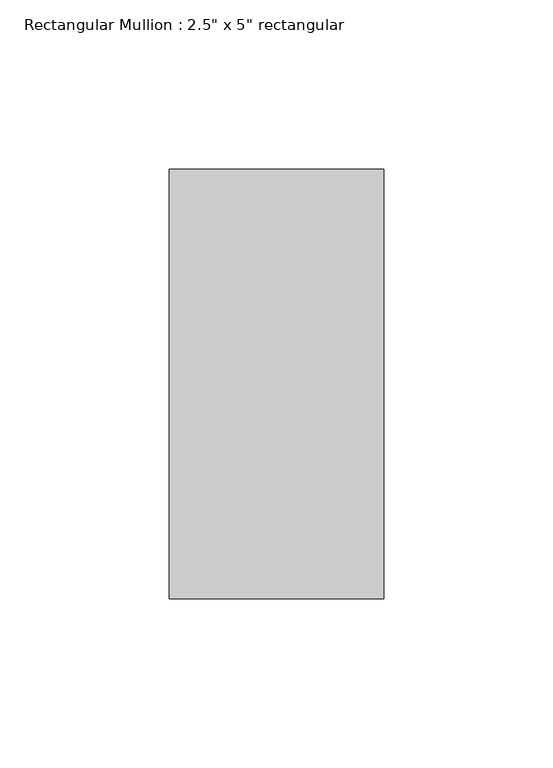
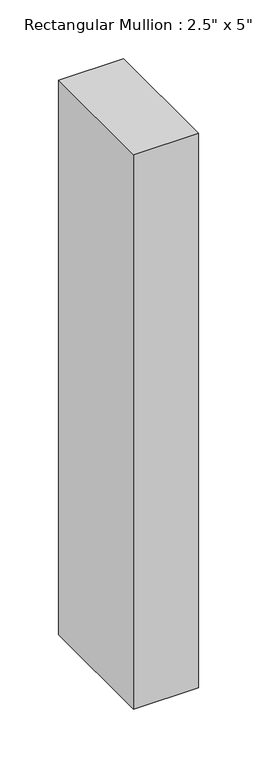
"""IFC4 building model written with IfcOpenShell, lengths in millimetres: member geometry."""

from ifc_helpers import new_model, si_unit, frame, origin, place, context, project, spatial, polyline, outline, extrude, source, transform, mapped, element, save


def member_cd3c8de8(model_context):
    return source(origin(), model_context, "Body", "SweptSolid", [
        extrude(outline(polyline([(0.0, 63.5), (0.0, -63.5), (-63.5, -63.5), (-63.5, 63.5), (0.0, 63.5)])), frame((0.0, 0.0, -574.3245158), z_axis=(0.0, 0.0, 1.0), x_axis=(1.0, 0.0, 0.0)), (0.0, 0.0, 1.0), 574.3245158),
    ])


if __name__ == "__main__":
    model = new_model("IFC4")
    model_context = context("Model", 3, world=origin())
    ifc_project = project(units=[si_unit("LENGTHUNIT", "METRE", prefix="MILLI")], contexts=[model_context])
    site = spatial("IfcSite", under=ifc_project)
    building = spatial("IfcBuilding", under=site)
    placement = place(None, origin())
    member_shape = member_cd3c8de8(model_context)
    element("IfcMember", 1, ObjectType="Rectangular Mullion : 2.5\" x 5\" rectangular", at=placement, inside=building, context=model_context, shape_type="MappedRepresentation", body=[
        mapped(member_shape, transform((0.0, 0.0, 0.0), x_axis=(1.0, 0.0, 0.0), y_axis=(0.0, 1.0, 0.0), z_axis=(0.0, 0.0, 1.0))),
    ])
    save(model, "model.ifc")

# Revit data of these elements
# Type "Rectangular Mullion : 2.5\" x 5\" rectangular"
#   built-in parameter 1007304 = 0.416667 (stored number, unit not read)
#   built-in parameter 1007301 = 0.104167 (stored number, unit not read)
#   built-in parameter 1007300 = 0.104167 (stored number, unit not read)
# Element 1 (IfcMember, "Rectangular Mullion : 2.5\" x 5\" rectangular")
#   Materials on its faces: "Aluminum"
# Materials
#   "Aluminum": class "Metal", colour RGB 247 247 247, transparency 0, Description = "Aluminum 6061", Cost = 0
